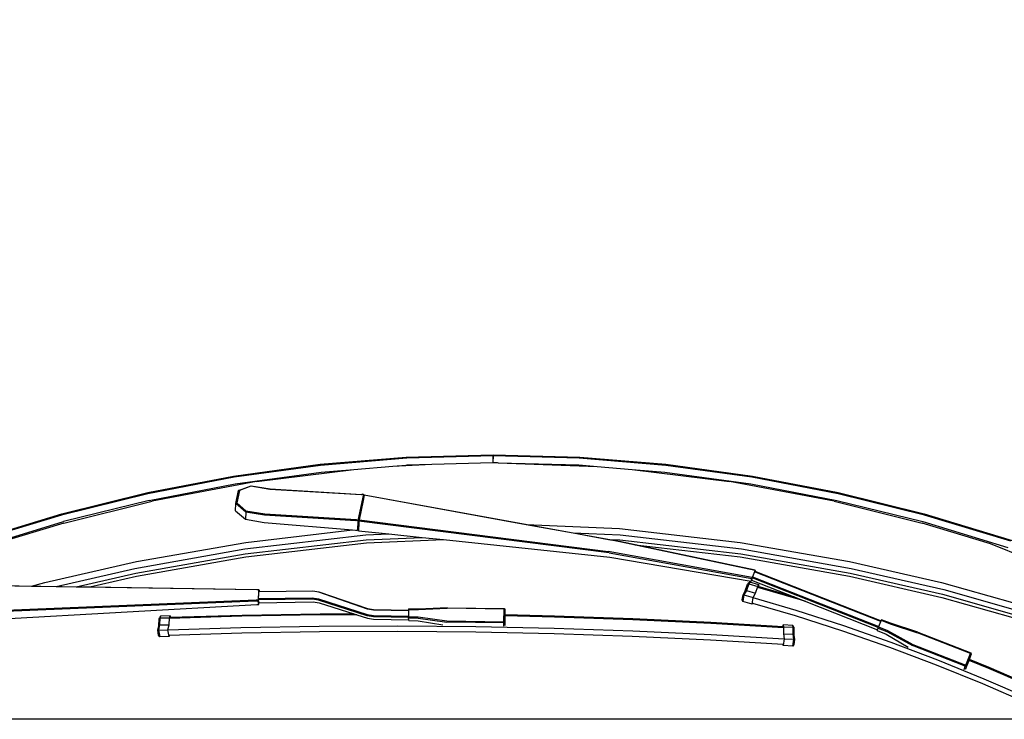
# Model space of a CAD drawing. Units: inches. Extents: x -4737294 to -4736756, y 1716389 to 1717040.
# Tile 13 of 25: x -4737171 to -4737127, y 1716601 to 1716633. Entities that reach past the tile are written whole.
import ezdxf

# ---------------------------------------------------------------- set-up
doc = ezdxf.new("R2010")
doc.units = ezdxf.units.IN
doc.header["$MEASUREMENT"] = 0
doc.layers.add('A-ANNO-DIMS', color=2, linetype='Continuous', lineweight=18)
doc.layers.add('A-EQPM-VEHI', color=250, linetype='Continuous', lineweight=13)
doc.layers.add('Edges', color=250, linetype='Continuous')
doc.styles.get("Standard").update_dxf_attribs({"font": 'arial.ttf'})
doc.dimstyles.get("Standard").update_dxf_attribs({"dimtxt": 8, "dimasz": 0.18, "dimexe": 0.18, "dimexo": 0.0625, "dimgap": 0.09, "dimtad": 0, "dimtih": 1, "dimtoh": 1, "dimzin": 0, "dimdsep": 46, "dimlunit": 3, "dimtxsty": 'Standard', "dimcen": 0.09, "dimadec": 0, "dimazin": 0, "dimtfac": 1, "dimtofl": 0, "dimtmove": 0, "dimatfit": 3, "dimfxl": 1, "dimtolj": 1, "dimtzin": 0, "dimarcsym": 0})

# ---------------------------------------------------------------- blocks, each defined once
blk = doc.blocks.new('Nissan Qashqai pl')
at = {"layer": 'Edges'}
for p, q in [((8.3852, 12.4994), (8.3608, 12.4393)), ((8.5103, 12.4859), (8.4895, 12.4381)), ((8.5112, 12.4856), (8.4904, 12.4377)), ((8.5222, 12.4807), (8.5014, 12.4329)), ((8.5062, 12.431), (8.5269, 12.4785)), ((8.3296, 12.3703), (8.3573, 12.4618)), ((8.3582, 12.4606), (8.3311, 12.3708)), ((8.4009, 12.3883), (8.4217, 12.4622)), ((8.4084, 12.3907), (8.4296, 12.4651)), ((8.4133, 12.3896), (8.4343, 12.4637)), ((8.4165, 12.3888), (8.4375, 12.4627)), ((8.3377, 12.3689), (8.3646, 12.4572)), ((8.3608, 12.4393), (8.3392, 12.3684)), ((8.3608, 12.4393), (8.3608, 12.4393)), ((8.4895, 12.4381), (8.4811, 12.4174)), ((8.5014, 12.4329), (8.4817, 12.3847)), ((8.4904, 12.4377), (8.482, 12.4171)), ((8.4866, 12.3829), (8.5062, 12.431)), ((8.4526, 12.3639), (8.4742, 12.4188)), ((8.4747, 12.4185), (8.4532, 12.3636)), ((8.4742, 12.4188), (8.4754, 12.4193)), ((8.4747, 12.4185), (8.4742, 12.4188)), ((8.4754, 12.4193), (8.4747, 12.4185)), ((8.4869, 12.4136), (8.4747, 12.4185)), ((8.4754, 12.4193), (8.4876, 12.4144)), ((8.4791, 12.4183), (8.4754, 12.4193)), ((8.4654, 12.3587), (8.4869, 12.4136)), ((8.4881, 12.4131), (8.4666, 12.3582)), ((8.4811, 12.4174), (8.4791, 12.4183)), ((8.482, 12.4171), (8.4811, 12.4174)), ((8.4912, 12.4133), (8.482, 12.4171)), ((8.4869, 12.4136), (8.4876, 12.4144)), ((8.4881, 12.4131), (8.4869, 12.4136)), ((8.4876, 12.4144), (8.4912, 12.4133)), ((8.4876, 12.4144), (8.4881, 12.4131)), ((8.4914, 12.4121), (8.4881, 12.4131)), ((8.4913, 12.4133), (8.4912, 12.4133)), ((8.4913, 12.4132), (8.4913, 12.4133)), ((8.3792, 12.2926), (8.4009, 12.3883)), ((8.3864, 12.2945), (8.4084, 12.3907)), ((8.3913, 12.2935), (8.4133, 12.3896)), ((8.3945, 12.2929), (8.4165, 12.3888)), ((8.4817, 12.3847), (8.4633, 12.3359)), ((8.4683, 12.3345), (8.4866, 12.3829)), ((8.3076, 12.281), (8.3296, 12.3703)), ((8.3311, 12.3708), (8.3089, 12.2811)), ((8.3157, 12.2795), (8.3377, 12.3689)), ((8.3166, 12.2767), (8.3392, 12.3684)), ((8.4526, 12.3639), (8.4434, 12.3353)), ((8.4439, 12.335), (8.4532, 12.3636)), ((8.4509, 12.3322), (8.4654, 12.3587)), ((8.4521, 12.3317), (8.4666, 12.3582)), ((8.4547, 12.3309), (8.4682, 12.3538)), ((8.4434, 12.3353), (8.4397, 12.326)), ((8.4403, 12.3257), (8.4439, 12.335)), ((8.4633, 12.3359), (8.4461, 12.2868)), ((8.4472, 12.3229), (8.4509, 12.3322)), ((8.4484, 12.3224), (8.4521, 12.3317)), ((8.4511, 12.3216), (8.4547, 12.3309)), ((8.4512, 12.2856), (8.4683, 12.3345)), ((8.3894, 12.1944), (8.4409, 12.3255)), ((8.4415, 12.3252), (8.3899, 12.1941)), ((8.3951, 12.192), (8.4467, 12.3231)), ((8.4479, 12.3226), (8.3963, 12.1915)), ((8.4209, 12.2475), (8.4502, 12.3219)), ((8.4403, 12.3257), (8.4397, 12.326)), ((8.4409, 12.3255), (8.4403, 12.3257)), ((8.4415, 12.3252), (8.4409, 12.3255)), ((8.4467, 12.3231), (8.4415, 12.3252)), ((8.4472, 12.3229), (8.4467, 12.3231)), ((8.4479, 12.3226), (8.4472, 12.3229)), ((8.4484, 12.3224), (8.4479, 12.3226)), ((8.4502, 12.3219), (8.4484, 12.3224)), ((8.4511, 12.3216), (8.4502, 12.3219)), ((8.3593, 12.1791), (8.3792, 12.2926)), ((8.3662, 12.1803), (8.3864, 12.2945)), ((8.3713, 12.1796), (8.3913, 12.2935)), ((8.3745, 12.1792), (8.3945, 12.2929)), ((8.4461, 12.2868), (8.4302, 12.2373)), ((8.4353, 12.2363), (8.4512, 12.2856)), ((8.2905, 12.1918), (8.3076, 12.281)), ((8.3089, 12.2811), (8.2916, 12.1913)), ((8.3166, 12.2767), (8.296, 12.168)), ((8.2985, 12.1901), (8.3157, 12.2795)), ((8.4163, 12.2359), (8.4209, 12.2475)), ((8.4209, 12.2475), (8.4191, 12.2418)), ((8.3986, 12.1908), (8.4163, 12.2359)), ((8.4163, 12.2359), (8.4052, 12.1979)), ((8.4191, 12.2418), (8.4061, 12.1973)), ((8.4302, 12.2373), (8.4171, 12.1926)), ((8.4224, 12.1919), (8.4353, 12.2363)), ((8.4475, 12.2348), (8.4457, 12.2337)), ((8.4475, 12.2348), (8.4484, 12.235)), ((8.4555, 12.2348), (8.4475, 12.2348)), ((8.4484, 12.235), (8.4557, 12.235)), ((8.46, 12.2348), (8.4549, 12.2341)), ((8.4557, 12.235), (8.4603, 12.2357)), ((8.4595, 12.2249), (8.46, 12.2348)), ((8.46, 12.2348), (8.4603, 12.2357)), ((8.4671, 12.2337), (8.46, 12.2348)), ((8.4603, 12.2357), (8.4655, 12.2348)), ((8.4655, 12.2348), (8.4671, 12.2337)), ((8.448, 12.2241), (8.4435, 12.1487)), ((8.4457, 12.2337), (8.4452, 12.2238)), ((8.4452, 12.2238), (8.4471, 12.2242)), ((8.4476, 12.2341), (8.4457, 12.2337)), ((8.4471, 12.2242), (8.4476, 12.2341)), ((8.4471, 12.2242), (8.4544, 12.2242)), ((8.4549, 12.2341), (8.4476, 12.2341)), ((8.4544, 12.2242), (8.4549, 12.2341)), ((8.4544, 12.2242), (8.4595, 12.2249)), ((8.4601, 12.2247), (8.4555, 12.1488)), ((8.4595, 12.2249), (8.4666, 12.2237)), ((8.4671, 12.2337), (8.4666, 12.2237)), ((8.4471, 12.2238), (8.4425, 12.1485)), ((8.4471, 12.2238), (8.4452, 12.2238)), ((8.4471, 12.2239), (8.4471, 12.2238)), ((8.4607, 12.1481), (8.4652, 12.2237)), ((8.4652, 12.2237), (8.4652, 12.2238)), ((8.4666, 12.2237), (8.4652, 12.2237)), ((8.3887, 12.1946), (8.3575, 12.0475)), ((8.3882, 12.1948), (8.3618, 12.07)), ((8.3887, 12.1946), (8.3882, 12.1948)), ((8.3882, 12.1948), (8.3894, 12.1944)), ((8.3894, 12.1944), (8.3887, 12.1946)), ((8.3894, 12.1944), (8.3894, 12.1944)), ((8.3894, 12.1944), (8.3899, 12.1941)), ((8.3899, 12.1941), (8.3951, 12.192)), ((8.4035, 12.1986), (8.4007, 12.189)), ((8.4023, 12.1879), (8.4052, 12.1975)), ((8.4052, 12.1975), (8.4035, 12.1986)), ((8.4035, 12.1986), (8.4052, 12.1979)), ((8.4052, 12.1979), (8.4052, 12.1978)), ((8.412, 12.195), (8.4052, 12.1975)), ((8.4092, 12.1855), (8.412, 12.195)), ((8.4167, 12.1925), (8.412, 12.195)), ((8.2781, 12.1018), (8.2905, 12.1918)), ((8.2916, 12.1913), (8.2793, 12.1016)), ((8.2862, 12.1008), (8.2985, 12.1901)), ((8.3957, 12.1917), (8.3688, 12.0419)), ((8.3702, 12.0427), (8.3969, 12.1913)), ((8.3746, 12.0435), (8.3995, 12.1905)), ((8.3951, 12.192), (8.3963, 12.1915)), ((8.3957, 12.1917), (8.3951, 12.192)), ((8.3969, 12.1913), (8.3957, 12.1917)), ((8.3963, 12.1915), (8.3986, 12.1908)), ((8.3995, 12.1905), (8.3969, 12.1913)), ((8.3995, 12.1905), (8.3986, 12.1908)), ((8.4007, 12.189), (8.4023, 12.1879)), ((8.4007, 12.189), (8.402, 12.1874)), ((8.4028, 12.1868), (8.402, 12.1874)), ((8.402, 12.1874), (8.4027, 12.1871)), ((8.4023, 12.1879), (8.4092, 12.1855)), ((8.4097, 12.1844), (8.4028, 12.1868)), ((8.4092, 12.1855), (8.4139, 12.1829)), ((8.4139, 12.1821), (8.4097, 12.1844)), ((8.4139, 12.1829), (8.4167, 12.1925)), ((8.4237, 12.1914), (8.4167, 12.1925)), ((8.4237, 12.1914), (8.4209, 12.1819)), ((8.4223, 12.1918), (8.4224, 12.1919)), ((8.4224, 12.1919), (8.4237, 12.1914)), ((8.3448, 12.0536), (8.3593, 12.1791)), ((8.3516, 12.0542), (8.3662, 12.1803)), ((8.3567, 12.0538), (8.3713, 12.1796)), ((8.3618, 12.07), (8.3745, 12.1792)), ((8.4139, 12.1829), (8.4209, 12.1819)), ((8.4139, 12.1821), (8.4139, 12.1829)), ((8.4191, 12.1813), (8.4139, 12.1821)), ((8.4209, 12.1819), (8.4191, 12.1813)), ((8.2834, 12.0669), (8.296, 12.168)), ((8.4425, 12.1485), (8.4387, 12.0674)), ((8.4435, 12.1487), (8.4397, 12.0674)), ((8.4555, 12.1488), (8.4517, 12.0674)), ((8.4568, 12.0669), (8.4607, 12.1481)), ((8.2708, 12.0123), (8.2781, 12.1018)), ((8.2793, 12.1016), (8.2719, 12.0118)), ((8.2834, 12.0669), (8.2862, 12.1008)), ((8.2804, 12.0305), (8.2834, 12.0669)), ((8.3618, 12.07), (8.3574, 12.0489)), ((8.4387, 12.0674), (8.4359, 11.9861)), ((8.4397, 12.0674), (8.4369, 11.9861)), ((8.4517, 12.0674), (8.4489, 11.9858)), ((8.4541, 11.9857), (8.4568, 12.0669)), ((8.3406, 11.9567), (8.3448, 12.0536)), ((8.3495, 12.0053), (8.3516, 12.0542)), ((8.3562, 12.0421), (8.3567, 12.0538)), ((8.3575, 12.0475), (8.3104, 11.7881)), ((8.336, 11.7828), (8.3688, 12.0419)), ((8.3702, 12.0427), (8.3374, 11.7826)), ((8.3495, 12.0053), (8.3562, 12.0421)), ((8.3562, 12.0421), (8.3574, 12.0489)), ((8.3565, 11.8707), (8.3746, 12.0435)), ((8.2765, 11.9273), (8.2804, 12.0305)), ((8.2788, 12.0114), (8.2804, 12.0305)), ((8.2682, 11.9221), (8.2708, 12.0123)), ((8.2719, 12.0118), (8.2695, 11.9221)), ((8.2765, 11.9273), (8.2788, 12.0114)), ((8.3406, 11.9567), (8.3495, 12.0053)), ((8.4359, 11.9861), (8.4348, 11.9346)), ((8.4369, 11.9861), (8.4358, 11.9346)), ((8.4489, 11.9858), (8.4471, 11.9043)), ((8.4523, 11.9043), (8.4541, 11.9857)), ((8.31, 11.7882), (8.3406, 11.9567)), ((8.2764, 11.9263), (8.2765, 11.9273)), ((8.4272, 11.8746), (8.4281, 11.9336)), ((8.4287, 11.9335), (8.4278, 11.8745)), ((8.4281, 11.9336), (8.429, 11.9345)), ((8.4281, 11.9336), (8.4287, 11.9336)), ((8.4287, 11.9335), (8.4281, 11.9336)), ((8.429, 11.9345), (8.4287, 11.9336)), ((8.4287, 11.9336), (8.4287, 11.9335)), ((8.4418, 11.9332), (8.4287, 11.9335)), ((8.4328, 11.9347), (8.429, 11.9345)), ((8.429, 11.9345), (8.4326, 11.9345)), ((8.4328, 11.9347), (8.4326, 11.9345)), ((8.4326, 11.9345), (8.4348, 11.9344)), ((8.4348, 11.9346), (8.4328, 11.9347)), ((8.4348, 11.9346), (8.4348, 11.9344)), ((8.4358, 11.9346), (8.4348, 11.9346)), ((8.4348, 11.9344), (8.4358, 11.9344)), ((8.4358, 11.9346), (8.4358, 11.9344)), ((8.4459, 11.9344), (8.4358, 11.9346)), ((8.4358, 11.9344), (8.4422, 11.9342)), ((8.441, 11.8742), (8.4418, 11.9332)), ((8.4418, 11.9332), (8.4422, 11.9342)), ((8.4431, 11.9332), (8.4418, 11.9332)), ((8.4422, 11.9342), (8.4459, 11.9344)), ((8.4422, 11.9342), (8.4431, 11.9332)), ((8.4431, 11.9332), (8.4422, 11.8742)), ((8.4464, 11.9334), (8.4431, 11.9332)), ((8.4459, 11.9344), (8.4459, 11.9344)), ((8.2708, 11.8319), (8.2682, 11.9221)), ((8.2763, 11.9223), (8.2695, 11.9221)), ((8.2695, 11.9221), (8.2763, 11.9219)), ((8.2695, 11.9221), (8.2719, 11.8323)), ((8.2763, 11.9223), (8.2764, 11.9263)), ((8.2763, 11.9219), (8.2763, 11.9223)), ((8.2781, 11.8585), (8.2763, 11.9219)), ((8.4471, 11.9043), (8.4464, 11.8227)), ((8.4516, 11.823), (8.4523, 11.9043)), ((8.3542, 11.8485), (8.3565, 11.8707)), ((8.3599, 11.7906), (8.3565, 11.8707)), ((8.4272, 11.8746), (8.4286, 11.8445)), ((8.4292, 11.8445), (8.4278, 11.8745)), ((8.4368, 11.8443), (8.441, 11.8742)), ((8.438, 11.8443), (8.4422, 11.8742)), ((8.4408, 11.8444), (8.4452, 11.8698)), ((8.28, 11.818), (8.2781, 11.8585)), ((8.2788, 11.8327), (8.2781, 11.8585)), ((8.2789, 11.8319), (8.2781, 11.8585)), ((8.3505, 11.8139), (8.3542, 11.8485)), ((8.3567, 11.7903), (8.3542, 11.8485)), ((8.4286, 11.8445), (8.4285, 11.8345)), ((8.4291, 11.8345), (8.4292, 11.8445)), ((8.4366, 11.8345), (8.4368, 11.8443)), ((8.4379, 11.8345), (8.438, 11.8443)), ((8.4406, 11.8344), (8.4408, 11.8444)), ((8.2781, 11.7423), (8.2708, 11.8319)), ((8.2719, 11.8323), (8.2793, 11.7426)), ((8.2789, 11.8319), (8.2788, 11.8327)), ((8.28, 11.818), (8.2789, 11.8319)), ((8.4291, 11.8345), (8.4285, 11.8345)), ((8.4298, 11.8345), (8.4291, 11.8345)), ((8.4292, 11.7978), (8.4298, 11.8345)), ((8.4304, 11.8345), (8.4298, 11.7978)), ((8.4304, 11.8345), (8.4298, 11.8345)), ((8.436, 11.8344), (8.4304, 11.8345)), ((8.4355, 11.7977), (8.436, 11.8344)), ((8.4366, 11.8343), (8.436, 11.8344)), ((8.4366, 11.8345), (8.4379, 11.8345)), ((8.4366, 11.8344), (8.4366, 11.8345)), ((8.4373, 11.8344), (8.4366, 11.8344)), ((8.4373, 11.8344), (8.4366, 11.8343)), ((8.4366, 11.8343), (8.4366, 11.8344)), ((8.4373, 11.8344), (8.4367, 11.7977)), ((8.4379, 11.8344), (8.4373, 11.8344)), ((8.4379, 11.8343), (8.4373, 11.8344)), ((8.4379, 11.8344), (8.4379, 11.8345)), ((8.4397, 11.8344), (8.4379, 11.8343)), ((8.4379, 11.8343), (8.4379, 11.8344)), ((8.4391, 11.7978), (8.4397, 11.8344)), ((8.4406, 11.8344), (8.4397, 11.8344)), ((8.2834, 11.7773), (8.28, 11.818)), ((8.4464, 11.8227), (8.4468, 11.7413)), ((8.452, 11.7418), (8.4516, 11.823)), ((8.3472, 11.7821), (8.3505, 11.8139)), ((8.3516, 11.79), (8.3505, 11.8139)), ((8.4281, 11.7914), (8.4292, 11.7978)), ((8.4298, 11.7978), (8.4287, 11.7914)), ((8.4344, 11.7912), (8.4355, 11.7977)), ((8.4367, 11.7977), (8.4357, 11.7912)), ((8.4381, 11.7914), (8.4391, 11.7978)), ((8.3038, 11.6903), (8.3095, 11.7853)), ((8.3099, 11.7851), (8.3042, 11.6901)), ((8.3092, 11.7863), (8.3093, 11.7873)), ((8.3092, 11.7863), (8.3099, 11.7851)), ((8.3095, 11.7853), (8.3092, 11.7863)), ((8.3093, 11.7873), (8.3367, 11.7816)), ((8.3159, 11.7869), (8.3093, 11.7873)), ((8.31, 11.7882), (8.3104, 11.7881)), ((8.3104, 11.7881), (8.3159, 11.7869)), ((8.3159, 11.7869), (8.336, 11.7828)), ((8.3662, 11.6639), (8.3516, 11.79)), ((8.3713, 11.6645), (8.3567, 11.7903)), ((8.3745, 11.665), (8.3599, 11.7906)), ((8.4107, 11.7411), (8.4281, 11.7914)), ((8.4287, 11.7914), (8.4111, 11.741)), ((8.4179, 11.7406), (8.4344, 11.7912)), ((8.4357, 11.7912), (8.4193, 11.7407)), ((8.4347, 11.7805), (8.4381, 11.7914)), ((8.296, 11.6762), (8.2834, 11.7773)), ((8.2862, 11.7434), (8.2834, 11.7773)), ((8.3298, 11.6848), (8.3355, 11.7798)), ((8.3369, 11.7796), (8.3312, 11.6846)), ((8.3355, 11.7798), (8.3366, 11.7806)), ((8.336, 11.7828), (8.3374, 11.7826)), ((8.3367, 11.7816), (8.3366, 11.7806)), ((8.3366, 11.7806), (8.3369, 11.7796)), ((8.3367, 11.7816), (8.347, 11.7811)), ((8.3374, 11.7826), (8.3406, 11.7824)), ((8.3385, 11.6842), (8.3464, 11.7761)), ((8.3458, 11.7813), (8.3406, 11.7824)), ((8.3406, 11.7824), (8.3457, 11.7821)), ((8.3458, 11.7813), (8.3457, 11.7821)), ((8.3457, 11.7821), (8.3472, 11.7821)), ((8.347, 11.7811), (8.3458, 11.7813)), ((8.3464, 11.7761), (8.3467, 11.7791)), ((8.3593, 11.6651), (8.3464, 11.7761)), ((8.3467, 11.7791), (8.347, 11.7811)), ((8.4222, 11.7413), (8.4337, 11.7775)), ((8.4337, 11.7775), (8.4347, 11.7805)), ((8.4337, 11.7775), (8.4339, 11.7423)), ((8.4347, 11.7805), (8.4348, 11.7421)), ((8.2985, 11.654), (8.2862, 11.7434)), ((8.2905, 11.6524), (8.2781, 11.7423)), ((8.2793, 11.7426), (8.2916, 11.6528)), ((8.4097, 11.7348), (8.4107, 11.7411)), ((8.4104, 11.6791), (8.4097, 11.7348)), ((8.4111, 11.741), (8.41, 11.7346)), ((8.41, 11.7346), (8.4108, 11.6791)), ((8.417, 11.7342), (8.4179, 11.7406)), ((8.4177, 11.678), (8.417, 11.7342)), ((8.4193, 11.7407), (8.4183, 11.7343)), ((8.4183, 11.7343), (8.4191, 11.678)), ((8.4213, 11.735), (8.4222, 11.7413)), ((8.4221, 11.6787), (8.4213, 11.735)), ((8.4339, 11.7423), (8.4353, 11.6613)), ((8.4348, 11.7421), (8.4362, 11.661)), ((8.4468, 11.7413), (8.4482, 11.66)), ((8.4534, 11.6608), (8.452, 11.7418)), ((8.3005, 11.6706), (8.3038, 11.6903)), ((8.3042, 11.6901), (8.3009, 11.6704)), ((8.3264, 11.6652), (8.3298, 11.6848)), ((8.3312, 11.6846), (8.3278, 11.665)), ((8.3352, 11.6646), (8.3385, 11.6842)), ((8.296, 11.6762), (8.3166, 11.5675)), ((8.4086, 11.6764), (8.4045, 11.4011)), ((8.4056, 11.5028), (8.4082, 11.6766)), ((8.4082, 11.6785), (8.4104, 11.6791)), ((8.4082, 11.6785), (8.4086, 11.6784)), ((8.4082, 11.6766), (8.4082, 11.6785)), ((8.4086, 11.6784), (8.4086, 11.6764)), ((8.4086, 11.6784), (8.4117, 11.6782)), ((8.4104, 11.6791), (8.4108, 11.6791)), ((8.4104, 11.6786), (8.4104, 11.6791)), ((8.4108, 11.6786), (8.4104, 11.6786)), ((8.4104, 11.6786), (8.4108, 11.6784)), ((8.4108, 11.6791), (8.4108, 11.6786)), ((8.4108, 11.6786), (8.4108, 11.6784)), ((8.4108, 11.6784), (8.4117, 11.6783)), ((8.4117, 11.6783), (8.4117, 11.6782)), ((8.4117, 11.6783), (8.4177, 11.678)), ((8.4117, 11.6782), (8.419, 11.6778)), ((8.4177, 11.678), (8.4191, 11.678)), ((8.419, 11.6778), (8.4203, 11.6778)), ((8.419, 11.6758), (8.419, 11.6778)), ((8.4305, 11.3996), (8.419, 11.6758)), ((8.4191, 11.678), (8.4221, 11.6787)), ((8.4238, 11.6786), (8.4203, 11.6778)), ((8.4203, 11.6778), (8.4204, 11.6758)), ((8.4204, 11.6758), (8.4319, 11.3996)), ((8.4238, 11.6786), (8.4221, 11.6787)), ((8.4238, 11.6766), (8.4238, 11.6786)), ((8.4394, 11.4014), (8.4238, 11.6766)), ((8.3053, 11.6574), (8.3005, 11.6706)), ((8.3009, 11.6704), (8.3054, 11.6583)), ((8.3182, 11.6557), (8.3264, 11.6652)), ((8.3278, 11.665), (8.319, 11.6546)), ((8.3264, 11.6542), (8.3352, 11.6646)), ((8.3278, 11.665), (8.3352, 11.6646)), ((8.3792, 11.5515), (8.3593, 11.6651)), ((8.3864, 11.5497), (8.3662, 11.6639)), ((8.3913, 11.5506), (8.3713, 11.6645)), ((8.3945, 11.5513), (8.3745, 11.665)), ((8.4353, 11.6613), (8.4375, 11.5863)), ((8.4362, 11.661), (8.4385, 11.5858)), ((8.3076, 11.5631), (8.2905, 11.6524)), ((8.2916, 11.6528), (8.3089, 11.5631)), ((8.3157, 11.5647), (8.2985, 11.654)), ((8.3054, 11.6583), (8.3053, 11.6574)), ((8.319, 11.6546), (8.3053, 11.6574)), ((8.3054, 11.6583), (8.3182, 11.6557)), ((8.319, 11.6546), (8.3182, 11.6557)), ((8.3264, 11.6542), (8.319, 11.6546)), ((8.4482, 11.66), (8.4505, 11.5843)), ((8.4557, 11.5855), (8.4534, 11.6608)), ((8.4377, 11.5857), (8.4357, 11.5864)), ((8.4357, 11.5864), (8.4359, 11.5765)), ((8.4357, 11.5864), (8.4375, 11.5863)), ((8.4375, 11.5863), (8.4375, 11.5862)), ((8.4379, 11.5758), (8.4377, 11.5857)), ((8.445, 11.5853), (8.4377, 11.5857)), ((8.4452, 11.5754), (8.445, 11.5853)), ((8.4503, 11.5841), (8.445, 11.5853)), ((8.4572, 11.5854), (8.4503, 11.5841)), ((8.4505, 11.5742), (8.4503, 11.5841)), ((8.4557, 11.5855), (8.4572, 11.5854)), ((8.4557, 11.5853), (8.4557, 11.5855)), ((8.4572, 11.5854), (8.4574, 11.5755)), ((8.4359, 11.5765), (8.4379, 11.5758)), ((8.4359, 11.5765), (8.4377, 11.5753)), ((8.4387, 11.5749), (8.4377, 11.5753)), ((8.4379, 11.5758), (8.4452, 11.5754)), ((8.4384, 11.5752), (8.4457, 11.5749)), ((8.446, 11.5746), (8.4387, 11.5749)), ((8.4452, 11.5754), (8.4505, 11.5742)), ((8.4507, 11.5734), (8.446, 11.5746)), ((8.4505, 11.5742), (8.4574, 11.5755)), ((8.4507, 11.5734), (8.4505, 11.5742)), ((8.4559, 11.5744), (8.4507, 11.5734)), ((8.4574, 11.5755), (8.4559, 11.5744)), ((8.3296, 11.4739), (8.3076, 11.5631)), ((8.3089, 11.5631), (8.3311, 11.4733)), ((8.3157, 11.5647), (8.3377, 11.4753)), ((8.3392, 11.4758), (8.3166, 11.5675)), ((8.4009, 11.4559), (8.3792, 11.5515)), ((8.4051, 11.4678), (8.3864, 11.5497)), ((8.4054, 11.4887), (8.3913, 11.5506)), ((8.4056, 11.5028), (8.3945, 11.5513)), ((8.4054, 11.4887), (8.4056, 11.5028)), ((8.4051, 11.4678), (8.4054, 11.4887)), ((8.3573, 11.3824), (8.3296, 11.4739)), ((8.3311, 11.4733), (8.3582, 11.3836)), ((8.3648, 11.3863), (8.3377, 11.4753)), ((8.3392, 11.4758), (8.3608, 11.4048)), ((8.4048, 11.4423), (8.4051, 11.4678)), ((8.4048, 11.4423), (8.4009, 11.4559)), ((8.4041, 11.4013), (8.4048, 11.4423))]:
    blk.add_line(p, q, dxfattribs=at)
blk = doc.blocks.new('car')
blk.add_blockref('Nissan Qashqai pl', (-9.7433, -11.9151))
blk = doc.blocks.new('*D63')
at = {"layer": 'A-ANNO-DIMS', "color": 0, "lineweight": -2, "transparency": 16777216}
for p, q in [((-4737062.207, 1716647.493), (-4737270.324, 1716647.493)), ((-4737270.144, 1716647.313), (-4737270.144, 1716628.418)), ((-4737270.144, 1716601.064), (-4737270.144, 1716619.959)), ((-4737062.207, 1716600.884), (-4737270.324, 1716600.884))]:
    blk.add_line(p, q, dxfattribs=at)
at = {"layer": 'A-ANNO-DIMS', "color": 0, "transparency": 16777216}
for points in [[(-4737270.174, 1716647.313), (-4737270.114, 1716647.313), (-4737270.144, 1716647.493)], [(-4737270.174, 1716601.064), (-4737270.114, 1716601.064), (-4737270.144, 1716600.884)]]:
    blk.add_solid(points, dxfattribs=at)
at = {"layer": 'Defpoints', "color": 0, "transparency": 16777216}
for p in [(-4737270.144, 1716647.493), (-4737062.144, 1716647.493), (-4737062.144, 1716600.884)]:
    blk.add_point(p, dxfattribs=at)
at = {"layer": 'A-ANNO-DIMS', "color": 0, "transparency": 16777216, "insert": (-4737270.144, 1716624.188), "char_height": 8, "attachment_point": 5}
blk.add_mtext('\\A1;3\'-10 1/2"', dxfattribs=at)

msp = doc.modelspace()

# ---------------------------------------------------------------- block references
at = {"layer": 'A-EQPM-VEHI', "xscale": 43.56002006885659, "yscale": 43.56002006885659, "zscale": 43.56002006885659, "rotation": 270}
msp.add_blockref('car', (-4737150.017, 1716548.61), dxfattribs=at)

# ---------------------------------------------------------------- dimensions: what is measured, and where the dimension line sits
at = {"layer": 'A-ANNO-DIMS'}
dim = msp.add_linear_dim(base=(-4737270.144, 1716647.493), p1=(-4737062.144, 1716600.884), p2=(-4737062.144, 1716647.493), angle=90, dimstyle='Standard', override={"dimdec": 1, "dimlfac": 1, "dimrnd": 0, "dimzin": 1, "dimdsep": 46, "dimlunit": 4, "dimfrac": 2}, dxfattribs=at)
dim.commit()
dim.dimension.update_dxf_attribs({"geometry": '*D63', "text_midpoint": (-4737270.144, 1716624.188)})

doc.saveas('drawing.dxf')
